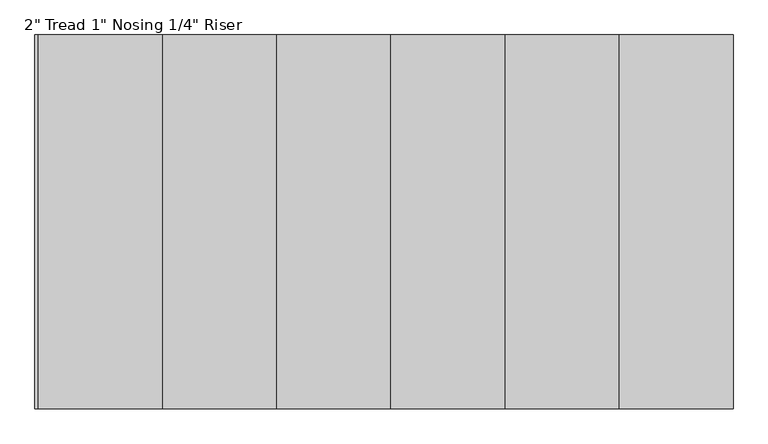
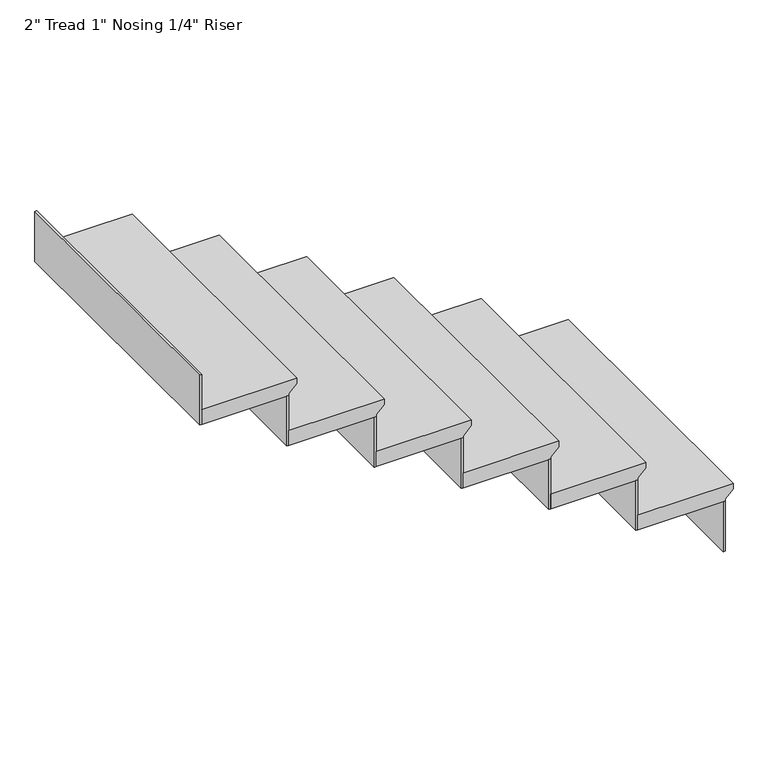
"""IFC4 building model written with IfcOpenShell, lengths in millimetres: stair flight geometry."""

from ifc_helpers import new_model, si_unit, frame, origin, place, context, project, spatial, polyline, outline, extrude, source, transform, mapped, element, save


def stair_flight_bf40378d(model_context):
    return source(origin(), model_context, "Body", "SweptSolid", [
        extrude(outline(polyline([(5080.0, -6841.3260609), (5080.0, -7146.1260609), (5029.2, -7146.1260609), (5029.2, -6866.7260609), (5035.55, -6866.7260609), (5060.95, -6841.3260609), (5080.0, -6841.3260609)])), frame((0.0, -7553.4810793, 0.0), z_axis=(0.0, 1.0, 0.0), x_axis=(0.0, 0.0, 1.0)), (0.0, 0.0, 1.0), 914.4),
        extrude(outline(polyline([(-6873.0760609, -6639.0810793), (-6866.7260609, -6639.0810793), (-6866.7260609, -7553.4810793), (-6873.0760609, -7553.4810793), (-6873.0760609, -6639.0810793)])), frame((0.0, 0.0, 4859.8666667), z_axis=(0.0, 0.0, 1.0), x_axis=(1.0, 0.0, 0.0)), (0.0, 0.0, 1.0), 169.3333333),
        extrude(outline(polyline([(-7152.4760609, -6639.0810793), (-7146.1260609, -6639.0810793), (-7146.1260609, -7553.4810793), (-7152.4760609, -7553.4810793), (-7152.4760609, -6639.0810793)])), frame((0.0, 0.0, 5029.2), z_axis=(0.0, 0.0, 1.0), x_axis=(1.0, 0.0, 0.0)), (0.0, 0.0, 1.0), 169.3333333),
        extrude(outline(polyline([(5249.3333333, -7120.7260609), (5249.3333333, -7425.5260609), (5198.5333333, -7425.5260609), (5198.5333333, -7146.1260609), (5204.8833333, -7146.1260609), (5230.2833333, -7120.7260609), (5249.3333333, -7120.7260609)])), frame((0.0, -7553.4810793, 0.0), z_axis=(0.0, 1.0, 0.0), x_axis=(0.0, 0.0, 1.0)), (0.0, 0.0, 1.0), 914.4),
        extrude(outline(polyline([(-7431.8760609, -6639.0810793), (-7425.5260609, -6639.0810793), (-7425.5260609, -7553.4810793), (-7431.8760609, -7553.4810793), (-7431.8760609, -6639.0810793)])), frame((0.0, 0.0, 5198.5333333), z_axis=(0.0, 0.0, 1.0), x_axis=(1.0, 0.0, 0.0)), (0.0, 0.0, 1.0), 169.3333333),
        extrude(outline(polyline([(5418.6666667, -7400.1260609), (5418.6666667, -7704.9260609), (5367.8666667, -7704.9260609), (5367.8666667, -7425.5260609), (5374.2166667, -7425.5260609), (5399.6166667, -7400.1260609), (5418.6666667, -7400.1260609)])), frame((0.0, -7553.4810793, 0.0), z_axis=(0.0, 1.0, 0.0), x_axis=(0.0, 0.0, 1.0)), (0.0, 0.0, 1.0), 914.4),
        extrude(outline(polyline([(-7711.2760609, -6639.0810793), (-7704.9260609, -6639.0810793), (-7704.9260609, -7553.4810793), (-7711.2760609, -7553.4810793), (-7711.2760609, -6639.0810793)])), frame((0.0, 0.0, 5367.8666667), z_axis=(0.0, 0.0, 1.0), x_axis=(1.0, 0.0, 0.0)), (0.0, 0.0, 1.0), 169.3333333),
        extrude(outline(polyline([(5588.0, -7679.5260609), (5588.0, -7984.3260609), (5537.2, -7984.3260609), (5537.2, -7704.9260609), (5543.55, -7704.9260609), (5568.95, -7679.5260609), (5588.0, -7679.5260609)])), frame((0.0, -7553.4810793, 0.0), z_axis=(0.0, 1.0, 0.0), x_axis=(0.0, 0.0, 1.0)), (0.0, 0.0, 1.0), 914.4),
        extrude(outline(polyline([(-7990.6760609, -6639.0810793), (-7984.3260609, -6639.0810793), (-7984.3260609, -7553.4810793), (-7990.6760609, -7553.4810793), (-7990.6760609, -6639.0810793)])), frame((0.0, 0.0, 5537.2), z_axis=(0.0, 0.0, 1.0), x_axis=(1.0, 0.0, 0.0)), (0.0, 0.0, 1.0), 169.3333333),
        extrude(outline(polyline([(5757.3333333, -7958.9260609), (5757.3333333, -8263.7260609), (5706.5333333, -8263.7260609), (5706.5333333, -7984.3260609), (5712.8833333, -7984.3260609), (5738.2833333, -7958.9260609), (5757.3333333, -7958.9260609)])), frame((0.0, -7553.4810793, 0.0), z_axis=(0.0, 1.0, 0.0), x_axis=(0.0, 0.0, 1.0)), (0.0, 0.0, 1.0), 914.4),
        extrude(outline(polyline([(-8270.0760609, -6639.0810793), (-8263.7260609, -6639.0810793), (-8263.7260609, -7553.4810793), (-8270.0760609, -7553.4810793), (-8270.0760609, -6639.0810793)])), frame((0.0, 0.0, 5706.5333333), z_axis=(0.0, 0.0, 1.0), x_axis=(1.0, 0.0, 0.0)), (0.0, 0.0, 1.0), 169.3333333),
        extrude(outline(polyline([(-8549.4760609, -6639.0810793), (-8543.1260609, -6639.0810793), (-8543.1260609, -7553.4810793), (-8549.4760609, -7553.4810793), (-8549.4760609, -6639.0810793)])), frame((0.0, 0.0, 5875.8666667), z_axis=(0.0, 0.0, 1.0), x_axis=(1.0, 0.0, 0.0)), (0.0, 0.0, 1.0), 169.3333333),
        extrude(outline(polyline([(5926.6666667, -8238.3260609), (5926.6666667, -8543.1260609), (5875.8666667, -8543.1260609), (5875.8666667, -8263.7260609), (5882.2166667, -8263.7260609), (5907.6166667, -8238.3260609), (5926.6666667, -8238.3260609)])), frame((0.0, -7553.4810793, 0.0), z_axis=(0.0, 1.0, 0.0), x_axis=(0.0, 0.0, 1.0)), (0.0, 0.0, 1.0), 914.4),
    ])


if __name__ == "__main__":
    model = new_model("IFC4")
    model_context = context("Model", 3, world=origin())
    ifc_project = project(units=[si_unit("LENGTHUNIT", "METRE", prefix="MILLI")], contexts=[model_context])
    site = spatial("IfcSite", under=ifc_project)
    building = spatial("IfcBuilding", under=site)
    placement = place(None, origin())
    stair_flight_shape = stair_flight_bf40378d(model_context)
    element("IfcStairFlight", 1, ObjectType="2\" Tread 1\" Nosing 1/4\" Riser", at=placement, inside=building, context=model_context, shape_type="MappedRepresentation", body=[
        mapped(stair_flight_shape, transform((0.0, 0.0, 0.0), x_axis=(1.0, 0.0, 0.0), y_axis=(0.0, 1.0, 0.0), z_axis=(0.0, 0.0, 1.0))),
    ])
    save(model, "model.ifc")
